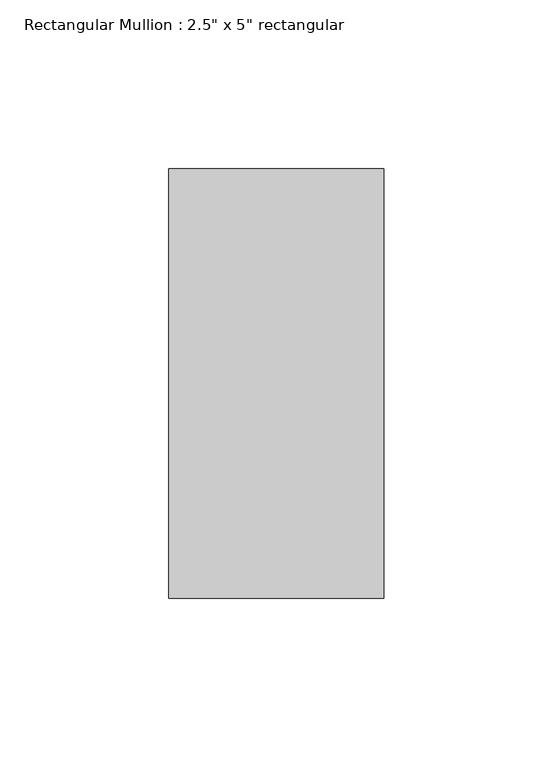
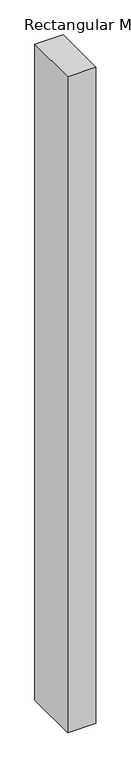
"""IFC4 building model written with IfcOpenShell, lengths in millimetres: member geometry."""

from ifc_helpers import new_model, si_unit, frame, origin, place, context, project, spatial, polyline, outline, extrude, source, transform, mapped, element, save


def member_eb14d2b7(model_context):
    return source(origin(), model_context, "Body", "SweptSolid", [
        extrude(outline(polyline([(0.0, 63.5), (0.0, -63.5), (-63.5, -63.5), (-63.5, 63.5), (0.0, 63.5)])), frame((0.0, 0.0, -1557.357611), z_axis=(0.0, 0.0, 1.0), x_axis=(1.0, 0.0, 0.0)), (0.0, 0.0, 1.0), 1557.357611),
    ])


if __name__ == "__main__":
    model = new_model("IFC4")
    model_context = context("Model", 3, world=origin())
    ifc_project = project(units=[si_unit("LENGTHUNIT", "METRE", prefix="MILLI")], contexts=[model_context])
    site = spatial("IfcSite", under=ifc_project)
    building = spatial("IfcBuilding", under=site)
    placement = place(None, origin())
    member_shape = member_eb14d2b7(model_context)
    element("IfcMember", 1, ObjectType="Rectangular Mullion : 2.5\" x 5\" rectangular", at=placement, inside=building, context=model_context, shape_type="MappedRepresentation", body=[
        mapped(member_shape, transform((0.0, 0.0, 0.0), x_axis=(1.0, 0.0, 0.0), y_axis=(0.0, 1.0, 0.0), z_axis=(0.0, 0.0, 1.0))),
    ])
    save(model, "model.ifc")

# Revit data of these elements
# Type "Rectangular Mullion : 2.5\" x 5\" rectangular"
#   built-in parameter 1007304 = 0.416667 (stored number, unit not read)
#   built-in parameter 1007301 = 0.104167 (stored number, unit not read)
#   built-in parameter 1007300 = 0.104167 (stored number, unit not read)
# Element 1 (IfcMember, "Rectangular Mullion : 2.5\" x 5\" rectangular")
#   Materials on its faces: "Aluminum"
# Materials
#   "Aluminum": class "Metal", colour RGB 247 247 247, transparency 0, Description = "Aluminum 6061", Cost = 0
